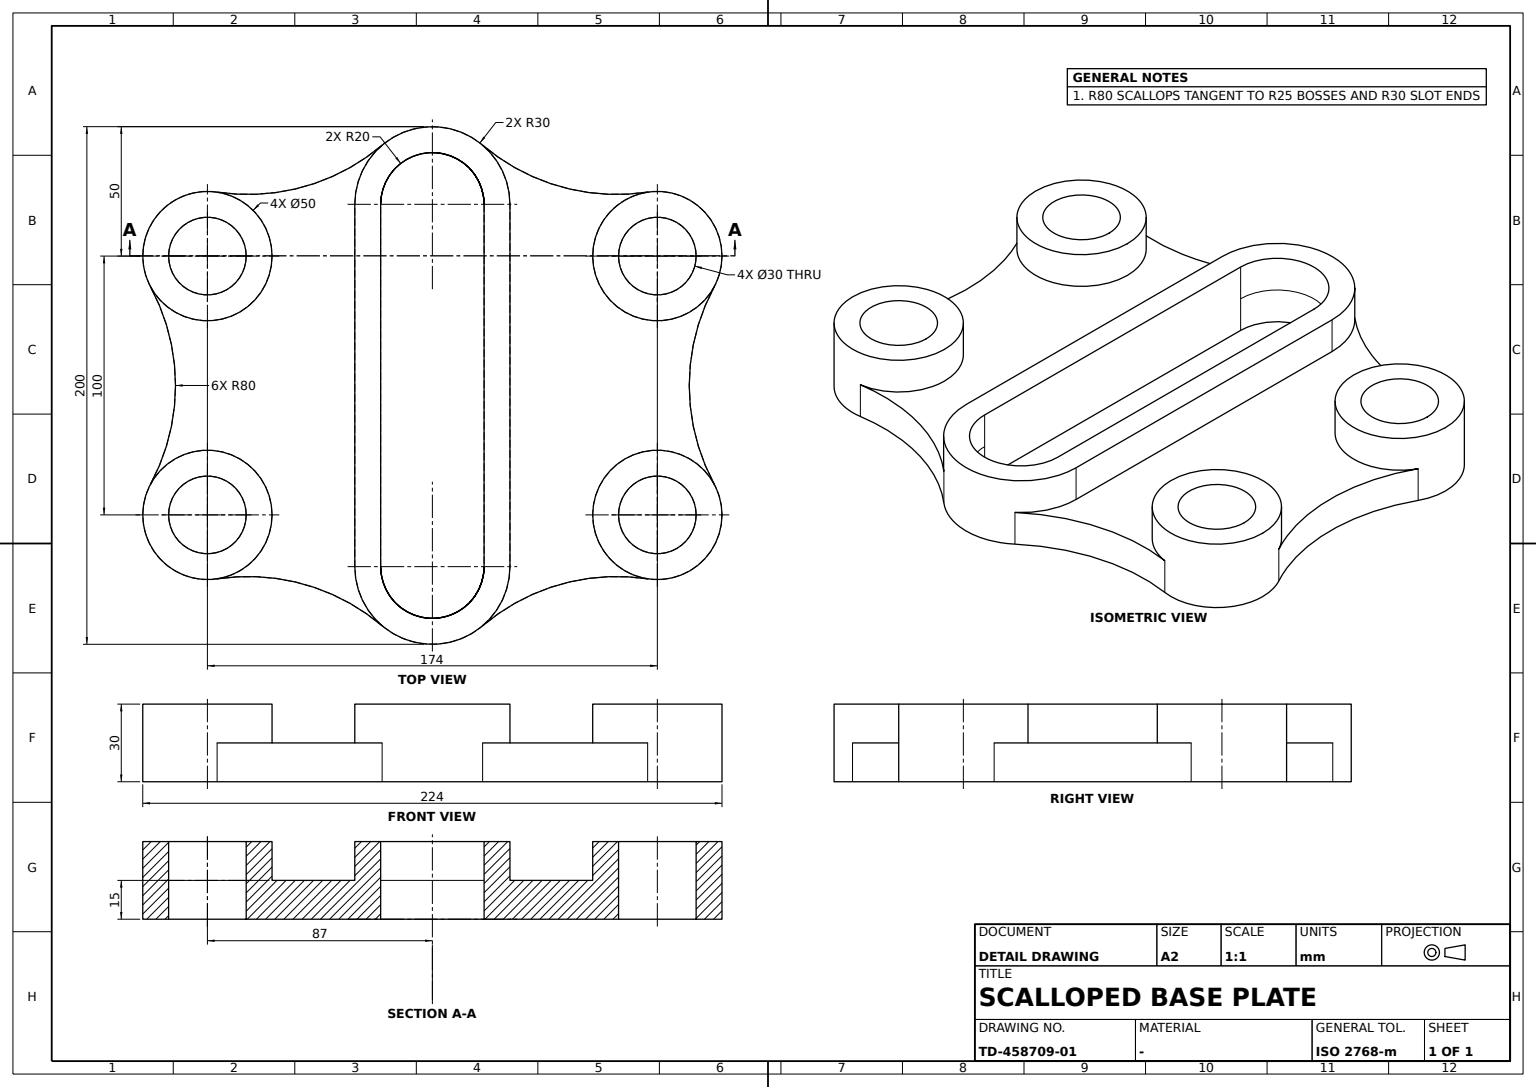
CATIA V5 part; units mm, degrees
sketch "Sketch1" plane through (0, 0, 0) normal (0, 0, 1) x (1, 0, 0)
  line L0 (0, 70) -> (0, -70) construction
  point P0 (0, 70)
  arc A0 (19.4302, -92.8576) -> (-19.4302, -92.8576) centre (0, -70) cw
  arc A1 (-19.4302, 92.8576) -> (19.4302, 92.8576) centre (0, 70) cw
  arc A2 (-83.2486, 74.7169) -> (-108.9836, 38.0952) centre (-87, 50) ccw
  point P1 (-87, 50)
  arc A3 (-108.9836, -38.0952) -> (-83.2486, -74.7169) centre (-87, -50) ccw
  point P2 (-87, -50)
  arc A4 (83.2486, -74.7169) -> (108.9836, -38.0952) centre (87, -50) ccw
  point P3 (87, -50)
  arc A5 (108.9836, 38.0952) -> (83.2486, 74.7169) centre (87, 50) ccw
  point P4 (87, 50)
  arc A6 (108.9836, 38.0952) -> (108.9836, -38.0952) centre (179.3309, 0) ccw
  point P5 (179.3309, 0)
  arc A7 (-108.9836, -38.0952) -> (-108.9836, 38.0952) centre (-179.3309, 0) ccw
  point P6 (-179.3309, 0)
  arc A8 (-83.2486, 74.7169) -> (-19.4302, 92.8576) centre (-71.2439, 153.8111) ccw
  arc A9 (19.4302, 92.8576) -> (83.2486, 74.7169) centre (71.2439, 153.8111) ccw
  arc A10 (-19.4302, -92.8576) -> (-83.2486, -74.7169) centre (-71.2439, -153.8111) ccw
  arc A11 (83.2486, -74.7169) -> (19.4302, -92.8576) centre (71.2439, -153.8111) ccw
  dimension "radius A1" = 30
  dimension "length L0" = 140
  dimension "distance x axis P0" = 70
  dimension "radius A0" = 30
  dimension "radius A2" = 25
  dimension "radius A3" = 25
  dimension "distance L0 P1" = 87
  dimension "distance P2 L0" = 87
  dimension "distance P1 P2" = 100
  dimension "distance P1 x axis" = 50
  dimension "radius A5" = 25
  dimension "radius A4" = 25
  dimension "distance P3 P4" = 100
  dimension "distance L0 P3" = 87
  dimension "distance P3 x axis" = 50
  dimension "distance P4 x axis" = 50
  dimension "radius A6" = 80
  dimension "radius A7" = 80
  dimension "radius A11" = 80
  dimension "radius A10" = 80
  dimension "radius A9" = 80
  dimension "radius A8" = 80
  constraint coincidence P0 y-axis
  constraint coincidence P5 x-axis
  constraint coincidence P6 x-axis
  constraint vertical L0 y-axis
  constraint tangency A6 A5
  constraint tangency A7 A3
  constraint tangency A9 A5
  constraint tangency A9 A1
  constraint tangency A8 A2
  constraint tangency A8 A1
  constraint tangency A11 A4
  constraint tangency A11 A0
  constraint tangency A10 A0
  constraint tangency A10 A3
extrude "Pad1" add sketch "Sketch1" against normal blind 15
sketch "Sketch2" plane through (0, 0, 0) normal (0, 0, 1) x (1, 0, 0)
  line L0 (0, 70) -> (0, -70) construction
  point P0 (0, 70)
  line L1 (30, 70) -> (30, -70)
  line L2 (-30, -70) -> (-30, 70)
  arc A0 (30, -70) -> (-30, -70) centre (0, -70) cw
  arc A1 (-30, 70) -> (30, 70) centre (0, 70) cw
  arc A2 (-19.4302, -92.8576) -> (19.4302, -92.8576) centre (0, -70) ccw construction
  arc A3 (19.4302, 92.8576) -> (-19.4302, 92.8576) centre (0, 70) ccw construction
  line L3 (0, 70) -> (0, -70) construction
  line L4 (20, 70) -> (20, -70)
  line L5 (-20, -70) -> (-20, 70)
  arc A4 (20, -70) -> (-20, -70) centre (0, -70) cw
  arc A5 (-20, 70) -> (20, 70) centre (0, 70) cw
  circle A6 centre (87, 50) radius 15
  circle A7 centre (87, 50) radius 25
  arc A8 (108.9836, 38.0952) -> (83.2486, 74.7169) centre (87, 50) ccw construction
  circle A9 centre (87, -50) radius 25
  circle A10 centre (87, -50) radius 15
  arc A11 (83.2486, -74.7169) -> (108.9836, -38.0952) centre (87, -50) ccw construction
  circle A12 centre (-87, 50) radius 25
  circle A13 centre (-87, 50) radius 15
  arc A14 (-83.2486, 74.7169) -> (-108.9836, 38.0952) centre (-87, 50) ccw construction
  circle A15 centre (-87, -50) radius 25
  circle A16 centre (-87, -50) radius 15
  arc A17 (-108.9836, -38.0952) -> (-83.2486, -74.7169) centre (-87, -50) ccw construction
  dimension "radius A1" = 30
  dimension "radius A5" = 20
  dimension "radius A4" = 20
  dimension "radius A6" = 15
  dimension "radius A7" = 25
  dimension "radius A9" = 25
  dimension "radius A10" = 15
  dimension "radius A12" = 25
  dimension "radius A13" = 15
  dimension "radius A15" = 25
  dimension "radius A16" = 15
  constraint coincidence P0 y-axis
  constraint coincidence A0 A2
  constraint vertical L0 y-axis
  constraint vertical L3 y-axis
  constraint tangency A0 L1
  constraint tangency A1 L1
  constraint tangency A0 L2
  constraint tangency A1 L2
  constraint tangency A4 L4
  constraint tangency A5 L4
  constraint tangency A4 L5
  constraint tangency A5 L5
  constraint concentricity A1 A3
  constraint concentricity A7 A8
  constraint concentricity A11 A9
  constraint concentricity A12 A14
  constraint concentricity A15 A17
extrude "Pad2" add sketch "Sketch2" along normal blind 15
sketch "Sketch3" plane through (0, 0, 0) normal (0, 0, 1) x (1, 0, 0)
  arc A0 (20, -70) -> (-20, -70) centre (0, -70) cw
  line L0 (20, 70) -> (20, -70)
  arc A1 (-20, 70) -> (20, 70) centre (0, 70) cw
  line L1 (-20, -70) -> (-20, 70)
  circle A2 centre (87, 50) radius 15
  circle A3 centre (87, -50) radius 15
  circle A4 centre (-87, 50) radius 15
  circle A5 centre (-87, -50) radius 15
extrude "Pocket1" cut sketch "Sketch3" against normal blind 15
